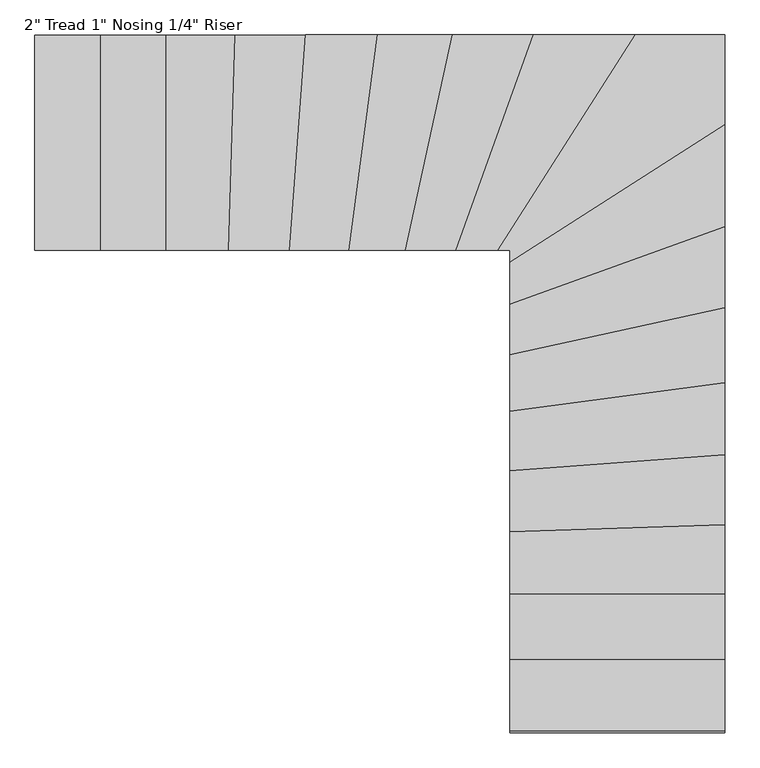
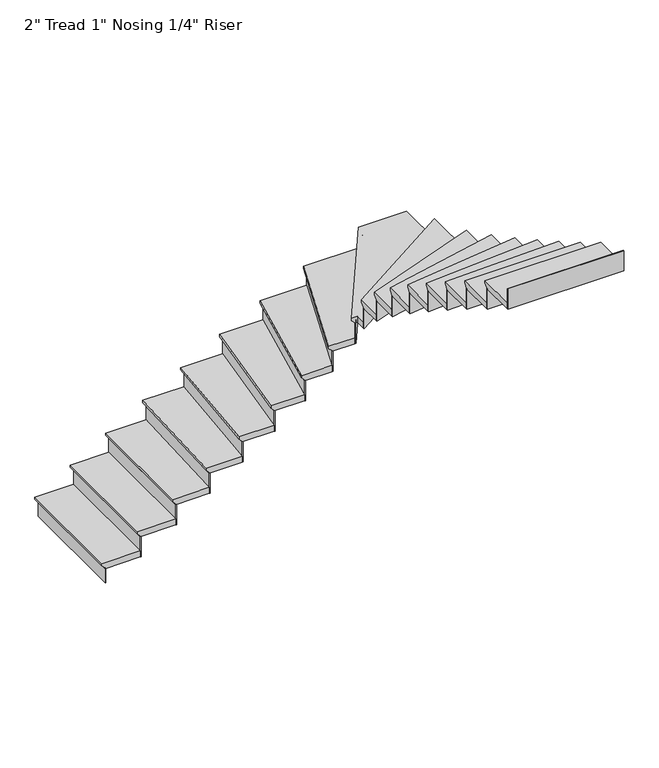
"""IFC4 building model written with IfcOpenShell, lengths in millimetres: stair flight geometry."""

from ifc_helpers import new_model, si_unit, origin, place, context, project, spatial, faceted_brep, source, transform, mapped, element, save


def stair_flight_aca28aa2(model_context):
    return source(origin(), model_context, "Body", "Brep", [
        faceted_brep([(-5670.2346501, 6411.0271763, 150.2833333), (-5670.2346501, 6411.0271763, 169.3333333), (-5670.2346501, 7325.4271763, 169.3333333), (-5670.2346501, 7325.4271763, 150.2833333), (-5644.8346501, 6411.0271763, 124.8833333), (-5644.8346501, 7325.4271763, 124.8833333), (-5365.4346501, 6411.0271763, 169.3333333), (-5365.4346501, 7325.4271763, 169.3333333), (-5644.8346501, 7325.4271763, 118.5333333), (-5365.4346501, 7325.4271763, 118.5333333), (-5365.4346501, 6411.0271763, 118.5333333), (-5644.8346501, 6411.0271763, 118.5333333)], [[[0, 1, 2, 3]], [[4, 0, 3, 5]], [[2, 1, 6, 7]], [[8, 9, 10, 11]], [[2, 7, 9, 8, 5, 3]], [[8, 11, 4, 5]], [[6, 1, 0, 4, 11, 10]], [[7, 6, 10, 9]]]),
        faceted_brep([(-5644.8346501, 6411.0271763, 118.5333333), (-5644.8346501, 6411.0271763, 0.0), (-5638.4846501, 6411.0271763, 0.0), (-5638.4846501, 6411.0271763, 118.5333333), (-5644.8346501, 7325.4271763, 118.5333333), (-5638.4846501, 7325.4271763, 118.5333333), (-5638.4846501, 7325.4271763, 0.0), (-5644.8346501, 7325.4271763, 0.0)], [[[0, 1, 2, 3]], [[4, 5, 6, 7]], [[1, 0, 4, 7]], [[2, 1, 7, 6]], [[3, 2, 6, 5]], [[0, 3, 5, 4]]]),
        faceted_brep([(-5365.4346501, 6411.0271763, 287.8666667), (-5365.4346501, 6411.0271763, 118.5333333), (-5359.0846501, 6411.0271763, 118.5333333), (-5359.0846501, 6411.0271763, 287.8666667), (-5365.4346501, 7325.4271763, 287.8666667), (-5359.0846501, 7325.4271763, 287.8666667), (-5359.0846501, 7325.4271763, 118.5333333), (-5365.4346501, 7325.4271763, 118.5333333)], [[[0, 1, 2, 3]], [[4, 5, 6, 7]], [[1, 0, 4, 7]], [[2, 1, 7, 6]], [[3, 2, 6, 5]], [[0, 3, 5, 4]]]),
        faceted_brep([(-5390.8346501, 7325.4271763, 338.6666667), (-5390.8346501, 6411.0271763, 338.6666667), (-5086.0346501, 6411.0271763, 338.6666667), (-5086.0346501, 7325.4271763, 338.6666667), (-5365.4346501, 7325.4271763, 287.8666667), (-5086.0346501, 7325.4271763, 287.8666667), (-5086.0346501, 6411.0271763, 287.8666667), (-5365.4346501, 6411.0271763, 287.8666667), (-5365.4346501, 7325.4271763, 294.2166667), (-5390.8346501, 7325.4271763, 319.6166667), (-5365.4346501, 6411.0271763, 294.2166667), (-5390.8346501, 6411.0271763, 319.6166667)], [[[0, 1, 2, 3]], [[4, 5, 6, 7]], [[0, 3, 5, 4, 8, 9]], [[4, 7, 10, 8]], [[2, 1, 11, 10, 7, 6]], [[3, 2, 6, 5]], [[11, 1, 0, 9]], [[10, 11, 9, 8]]]),
        faceted_brep([(-5086.0346501, 6411.0271763, 457.2), (-5086.0346501, 6411.0271763, 287.8666667), (-5079.6846501, 6411.0271763, 287.8666667), (-5079.6846501, 6411.0271763, 457.2), (-5086.0346501, 7325.4271763, 457.2), (-5079.6846501, 7325.4271763, 457.2), (-5079.6846501, 7325.4271763, 287.8666667), (-5086.0346501, 7325.4271763, 287.8666667)], [[[0, 1, 2, 3]], [[4, 5, 6, 7]], [[1, 0, 4, 7]], [[2, 1, 7, 6]], [[3, 2, 6, 5]], [[0, 3, 5, 4]]]),
        faceted_brep([(-5111.4346501, 7325.4271763, 508.0), (-5111.4346501, 6411.0271763, 508.0), (-4821.1765248, 6411.0271763, 508.0), (-4792.0670407, 7325.4271763, 508.0), (-5086.0346501, 7325.4271763, 457.2), (-4792.0670407, 7325.4271763, 457.2), (-4821.1765248, 6411.0271763, 457.2), (-5086.0346501, 6411.0271763, 457.2), (-5086.0346501, 7325.4271763, 463.55), (-5111.4346501, 7325.4271763, 488.95), (-5086.0346501, 6411.0271763, 463.55), (-5111.4346501, 6411.0271763, 488.95)], [[[0, 1, 2, 3]], [[4, 5, 6, 7]], [[0, 3, 5, 4, 8, 9]], [[4, 7, 10, 8]], [[2, 1, 11, 10, 7, 6]], [[3, 2, 6, 5]], [[11, 1, 0, 9]], [[10, 11, 9, 8]]]),
        faceted_brep([(-4821.1765248, 6411.0271763, 626.5333333), (-4821.1765248, 6411.0271763, 457.2), (-4814.823308, 6411.0271763, 457.2), (-4814.823308, 6411.0271763, 626.5333333), (-4792.0670407, 7325.4271763, 626.5333333), (-4785.7138239, 7325.4271763, 626.5333333), (-4785.7138239, 7325.4271763, 457.2), (-4792.0670407, 7325.4271763, 457.2)], [[[0, 1, 2, 3]], [[4, 5, 6, 7]], [[1, 0, 4, 7]], [[2, 1, 7, 6]], [[3, 2, 6, 5]], [[0, 3, 5, 4]]]),
        faceted_brep([(-4817.4799081, 7325.4271763, 677.3333333), (-4846.5893922, 6411.0271763, 677.3333333), (-4560.9843582, 6411.0271763, 677.3333333), (-4493.3461539, 7325.4271763, 677.3333333), (-4792.0670407, 7325.4271763, 626.5333333), (-4493.3461539, 7325.4271763, 626.5333333), (-4560.9843582, 6411.0271763, 626.5333333), (-4821.1765248, 6411.0271763, 626.5333333), (-4792.0670407, 7325.4271763, 632.8833333), (-4817.4799081, 7325.4271763, 658.2833333), (-4821.1765248, 6411.0271763, 632.8833333), (-4846.5893922, 6411.0271763, 658.2833333)], [[[0, 1, 2, 3]], [[4, 5, 6, 7]], [[0, 3, 5, 4, 8, 9]], [[4, 7, 10, 8]], [[2, 1, 11, 10, 7, 6]], [[3, 2, 6, 5]], [[11, 1, 0, 9]], [[10, 11, 9, 8]]]),
        faceted_brep([(-4560.9843582, 6411.0271763, 795.8666667), (-4560.9843582, 6411.0271763, 626.5333333), (-4554.6170096, 6411.0271763, 626.5333333), (-4554.6170096, 6411.0271763, 795.8666667), (-4493.3461539, 7325.4271763, 795.8666667), (-4486.9788054, 7325.4271763, 795.8666667), (-4486.9788054, 7325.4271763, 626.5333333), (-4493.3461539, 7325.4271763, 626.5333333)], [[[0, 1, 2, 3]], [[4, 5, 6, 7]], [[1, 0, 4, 7]], [[2, 1, 7, 6]], [[3, 2, 6, 5]], [[0, 3, 5, 4]]]),
        faceted_brep([(-4518.815548, 7325.4271763, 846.6666667), (-4586.4537523, 6411.0271763, 846.6666667), (-4308.1332907, 6411.0271763, 846.6666667), (-4187.0928787, 7325.4271763, 846.6666667), (-4493.3461539, 7325.4271763, 795.8666667), (-4187.0928787, 7325.4271763, 795.8666667), (-4308.1332907, 6411.0271763, 795.8666667), (-4560.9843582, 6411.0271763, 795.8666667), (-4493.3461539, 7325.4271763, 802.2166667), (-4518.815548, 7325.4271763, 827.6166667), (-4560.9843582, 6411.0271763, 802.2166667), (-4586.4537523, 6411.0271763, 827.6166667)], [[[0, 1, 2, 3]], [[4, 5, 6, 7]], [[0, 3, 5, 4, 8, 9]], [[4, 7, 10, 8]], [[2, 1, 11, 10, 7, 6]], [[3, 2, 6, 5]], [[11, 1, 0, 9]], [[10, 11, 9, 8]]]),
        faceted_brep([(-4308.1332907, 6411.0271763, 965.2), (-4308.1332907, 6411.0271763, 795.8666667), (-4301.7278994, 6411.0271763, 795.8666667), (-4301.7278994, 6411.0271763, 965.2), (-4187.0928787, 7325.4271763, 965.2), (-4180.6874873, 7325.4271763, 965.2), (-4180.6874873, 7325.4271763, 795.8666667), (-4187.0928787, 7325.4271763, 795.8666667)], [[[0, 1, 2, 3]], [[4, 5, 6, 7]], [[1, 0, 4, 7]], [[2, 1, 7, 6]], [[3, 2, 6, 5]], [[0, 3, 5, 4]]]),
        faceted_brep([(-4212.7144441, 7325.4271763, 1016.0), (-4333.7548562, 6411.0271763, 1016.0), (-4067.8285854, 6411.0271763, 1016.0), (-3867.8399188, 7325.4271763, 1016.0), (-4187.0928787, 7325.4271763, 965.2), (-3867.8399188, 7325.4271763, 965.2), (-4067.8285854, 6411.0271763, 965.2), (-4308.1332907, 6411.0271763, 965.2), (-4187.0928787, 7325.4271763, 971.55), (-4212.7144441, 7325.4271763, 996.95), (-4308.1332907, 6411.0271763, 971.55), (-4333.7548562, 6411.0271763, 996.95)], [[[0, 1, 2, 3]], [[4, 5, 6, 7]], [[0, 3, 5, 4, 8, 9]], [[4, 7, 10, 8]], [[2, 1, 11, 10, 7, 6]], [[3, 2, 6, 5]], [[11, 1, 0, 9]], [[10, 11, 9, 8]]]),
        faceted_brep([(-4067.8285854, 6411.0271763, 1134.5333333), (-4067.8285854, 6411.0271763, 965.2), (-4061.3284859, 6411.0271763, 965.2), (-4061.3284859, 6411.0271763, 1134.5333333), (-3867.8399188, 7325.4271763, 1134.5333333), (-3861.3398193, 7325.4271763, 1134.5333333), (-3861.3398193, 7325.4271763, 965.2), (-3867.8399188, 7325.4271763, 965.2)], [[[0, 1, 2, 3]], [[4, 5, 6, 7]], [[1, 0, 4, 7]], [[2, 1, 7, 6]], [[3, 2, 6, 5]], [[0, 3, 5, 4]]]),
        faceted_brep([(-3893.8403168, 7325.4271763, 1185.3333333), (-4093.8289834, 6411.0271763, 1185.3333333), (-3851.7328226, 6411.0271763, 1185.3333333), (-3523.1563179, 7325.4271763, 1185.3333333), (-3867.8399188, 7325.4271763, 1134.5333333), (-3523.1563179, 7325.4271763, 1134.5333333), (-3851.7328226, 6411.0271763, 1134.5333333), (-4067.8285854, 6411.0271763, 1134.5333333), (-3867.8399188, 7325.4271763, 1140.8833333), (-3893.8403168, 7325.4271763, 1166.2833333), (-4067.8285854, 6411.0271763, 1140.8833333), (-4093.8289834, 6411.0271763, 1166.2833333)], [[[0, 1, 2, 3]], [[4, 5, 6, 7]], [[0, 3, 5, 4, 8, 9]], [[4, 7, 10, 8]], [[2, 1, 11, 10, 7, 6]], [[3, 2, 6, 5]], [[11, 1, 0, 9]], [[10, 11, 9, 8]]]),
        faceted_brep([(-3851.7328226, 6411.0271763, 1303.8666667), (-3851.7328226, 6411.0271763, 1134.5333333), (-3844.9853027, 6411.0271763, 1134.5333333), (-3844.9853027, 6411.0271763, 1303.8666667), (-3523.1563179, 7325.4271763, 1303.8666667), (-3516.4087979, 7325.4271763, 1303.8666667), (-3516.4087979, 7325.4271763, 1134.5333333), (-3523.1563179, 7325.4271763, 1134.5333333)], [[[0, 1, 2, 3]], [[4, 5, 6, 7]], [[1, 0, 4, 7]], [[2, 1, 7, 6]], [[3, 2, 6, 5]], [[0, 3, 5, 4]]]),
        faceted_brep([(-3550.1463978, 7325.4271763, 1354.6666667), (-3878.7229025, 6411.0271763, 1354.6666667), (-3669.4620272, 6411.0271763, 1354.6666667), (-3084.8625918, 7325.4271763, 1354.6666667), (-3523.1563179, 7325.4271763, 1303.8666667), (-3084.8625918, 7325.4271763, 1303.8666667), (-3669.4620272, 6411.0271763, 1303.8666667), (-3851.7328226, 6411.0271763, 1303.8666667), (-3523.1563179, 7325.4271763, 1310.2166667), (-3550.1463978, 7325.4271763, 1335.6166667), (-3851.7328226, 6411.0271763, 1310.2166667), (-3878.7229025, 6411.0271763, 1335.6166667)], [[[0, 1, 2, 3]], [[4, 5, 6, 7]], [[0, 3, 5, 4, 8, 9]], [[4, 7, 10, 8]], [[2, 1, 11, 10, 7, 6]], [[3, 2, 6, 5]], [[11, 1, 0, 9]], [[10, 11, 9, 8]]]),
        faceted_brep([(-3669.4620272, 6411.0271763, 1473.2), (-3669.4620272, 6411.0271763, 1303.8666667), (-3661.9251968, 6411.0271763, 1303.8666667), (-3661.9251968, 6411.0271763, 1473.2), (-3084.8625918, 7325.4271763, 1473.2), (-3077.3257614, 7325.4271763, 1473.2), (-3077.3257614, 7325.4271763, 1303.8666667), (-3084.8625918, 7325.4271763, 1303.8666667)], [[[0, 1, 2, 3]], [[4, 5, 6, 7]], [[1, 0, 4, 7]], [[2, 1, 7, 6]], [[3, 2, 6, 5]], [[0, 3, 5, 4]]]),
        faceted_brep([(-2734.2976606, 6914.5676018, 1524.0), (-2734.2976606, 7325.4271763, 1524.0), (-3115.0099135, 7325.4271763, 1524.0), (-3699.6093489, 6411.0271763, 1524.0), (-3648.6976606, 6411.0271763, 1524.0), (-3648.6976606, 6329.9681664, 1524.0), (-2734.2976606, 7325.4271763, 1473.2), (-2734.2976606, 6914.5676018, 1473.2), (-3648.6976606, 6329.9681664, 1473.2), (-3648.6976606, 6411.0271763, 1473.2), (-3669.4620272, 6411.0271763, 1473.2), (-3084.8625918, 7325.4271763, 1473.2), (-3084.8625918, 7325.4271763, 1479.55), (-3115.0099135, 7325.4271763, 1504.95), (-3669.4620272, 6411.0271763, 1479.55), (-3699.6093489, 6411.0271763, 1504.95)], [[[0, 1, 2, 3, 4, 5]], [[6, 7, 8, 9, 10, 11]], [[1, 0, 7, 6]], [[2, 1, 6, 11, 12, 13]], [[11, 10, 14, 12]], [[4, 3, 15, 14, 10, 9]], [[5, 4, 9, 8]], [[0, 5, 8, 7]], [[15, 3, 2, 13]], [[14, 15, 13, 12]]]),
        faceted_brep([(-3648.6976606, 6329.9681664, 1642.5333333), (-3648.6976606, 6329.9681664, 1473.2), (-3648.6976606, 6322.4313359, 1473.2), (-3648.6976606, 6322.4313359, 1642.5333333), (-2734.2976606, 6914.5676018, 1642.5333333), (-2734.2976606, 6907.0307714, 1642.5333333), (-2734.2976606, 6907.0307714, 1473.2), (-2734.2976606, 6914.5676018, 1473.2)], [[[0, 1, 2, 3]], [[4, 5, 6, 7]], [[1, 0, 4, 7]], [[2, 1, 7, 6]], [[3, 2, 6, 5]], [[0, 3, 5, 4]]]),
        faceted_brep([(-2734.2976606, 6944.7149234, 1693.3333333), (-3648.6976606, 6360.115488, 1693.3333333), (-3648.6976606, 6154.0118545, 1693.3333333), (-2734.2976606, 6482.5883593, 1693.3333333), (-2734.2976606, 6914.5676018, 1642.5333333), (-2734.2976606, 6482.5883593, 1642.5333333), (-3648.6976606, 6154.0118545, 1642.5333333), (-3648.6976606, 6329.9681664, 1642.5333333), (-2734.2976606, 6914.5676018, 1648.8833333), (-2734.2976606, 6944.7149234, 1674.2833333), (-3648.6976606, 6329.9681664, 1648.8833333), (-3648.6976606, 6360.115488, 1674.2833333)], [[[0, 1, 2, 3]], [[4, 5, 6, 7]], [[0, 3, 5, 4, 8, 9]], [[4, 7, 10, 8]], [[2, 1, 11, 10, 7, 6]], [[3, 2, 6, 5]], [[11, 1, 0, 9]], [[10, 11, 9, 8]]]),
        faceted_brep([(-3648.6976606, 6154.0118545, 1811.8666667), (-3648.6976606, 6154.0118545, 1642.5333333), (-3648.6976606, 6147.2643345, 1642.5333333), (-3648.6976606, 6147.2643345, 1811.8666667), (-2734.2976606, 6482.5883593, 1811.8666667), (-2734.2976606, 6475.8408393, 1811.8666667), (-2734.2976606, 6475.8408393, 1642.5333333), (-2734.2976606, 6482.5883593, 1642.5333333)], [[[0, 1, 2, 3]], [[4, 5, 6, 7]], [[1, 0, 4, 7]], [[2, 1, 7, 6]], [[3, 2, 6, 5]], [[0, 3, 5, 4]]]),
        faceted_brep([(-2734.2976606, 6509.5784392, 1862.6666667), (-3648.6976606, 6181.0019344, 1862.6666667), (-3648.6976606, 5939.8954554, 1862.6666667), (-2734.2976606, 6139.884122, 1862.6666667), (-2734.2976606, 6482.5883593, 1811.8666667), (-2734.2976606, 6139.884122, 1811.8666667), (-3648.6976606, 5939.8954554, 1811.8666667), (-3648.6976606, 6154.0118545, 1811.8666667), (-2734.2976606, 6482.5883593, 1818.2166667), (-2734.2976606, 6509.5784392, 1843.6166667), (-3648.6976606, 6154.0118545, 1818.2166667), (-3648.6976606, 6181.0019344, 1843.6166667)], [[[0, 1, 2, 3]], [[4, 5, 6, 7]], [[0, 3, 5, 4, 8, 9]], [[4, 7, 10, 8]], [[2, 1, 11, 10, 7, 6]], [[3, 2, 6, 5]], [[11, 1, 0, 9]], [[10, 11, 9, 8]]]),
        faceted_brep([(-3648.6976606, 5939.8954554, 1981.2), (-3648.6976606, 5939.8954554, 1811.8666667), (-3648.6976606, 5933.3953559, 1811.8666667), (-3648.6976606, 5933.3953559, 1981.2), (-2734.2976606, 6139.884122, 1981.2), (-2734.2976606, 6133.3840225, 1981.2), (-2734.2976606, 6133.3840225, 1811.8666667), (-2734.2976606, 6139.884122, 1811.8666667)], [[[0, 1, 2, 3]], [[4, 5, 6, 7]], [[1, 0, 4, 7]], [[2, 1, 7, 6]], [[3, 2, 6, 5]], [[0, 3, 5, 4]]]),
        faceted_brep([(-2734.2976606, 6165.8845201, 2032.0), (-3648.6976606, 5965.8958535, 2032.0), (-3648.6976606, 5700.3484153, 2032.0), (-2734.2976606, 5821.3888274, 2032.0), (-2734.2976606, 6139.884122, 1981.2), (-2734.2976606, 5821.3888274, 1981.2), (-3648.6976606, 5700.3484153, 1981.2), (-3648.6976606, 5939.8954554, 1981.2), (-2734.2976606, 6139.884122, 1987.55), (-2734.2976606, 6165.8845201, 2012.95), (-3648.6976606, 5939.8954554, 1987.55), (-3648.6976606, 5965.8958535, 2012.95)], [[[0, 1, 2, 3]], [[4, 5, 6, 7]], [[0, 3, 5, 4, 8, 9]], [[4, 7, 10, 8]], [[2, 1, 11, 10, 7, 6]], [[3, 2, 6, 5]], [[11, 1, 0, 9]], [[10, 11, 9, 8]]]),
        faceted_brep([(-3648.6976606, 5700.3484153, 2150.5333333), (-3648.6976606, 5700.3484153, 1981.2), (-3648.6976606, 5693.9430239, 1981.2), (-3648.6976606, 5693.9430239, 2150.5333333), (-2734.2976606, 5821.3888274, 2150.5333333), (-2734.2976606, 5814.983436, 2150.5333333), (-2734.2976606, 5814.983436, 1981.2), (-2734.2976606, 5821.3888274, 1981.2)], [[[0, 1, 2, 3]], [[4, 5, 6, 7]], [[1, 0, 4, 7]], [[2, 1, 7, 6]], [[3, 2, 6, 5]], [[0, 3, 5, 4]]]),
        faceted_brep([(-2734.2976606, 5847.0103928, 2201.3333333), (-3648.6976606, 5725.9699807, 2201.3333333), (-3648.6976606, 5447.8016905, 2201.3333333), (-2734.2976606, 5515.4398948, 2201.3333333), (-2734.2976606, 5821.3888274, 2150.5333333), (-2734.2976606, 5515.4398948, 2150.5333333), (-3648.6976606, 5447.8016905, 2150.5333333), (-3648.6976606, 5700.3484153, 2150.5333333), (-2734.2976606, 5821.3888274, 2156.8833333), (-2734.2976606, 5847.0103928, 2182.2833333), (-3648.6976606, 5700.3484153, 2156.8833333), (-3648.6976606, 5725.9699807, 2182.2833333)], [[[0, 1, 2, 3]], [[4, 5, 6, 7]], [[0, 3, 5, 4, 8, 9]], [[4, 7, 10, 8]], [[2, 1, 11, 10, 7, 6]], [[3, 2, 6, 5]], [[11, 1, 0, 9]], [[10, 11, 9, 8]]]),
        faceted_brep([(-3648.6976606, 5447.8016905, 2319.8666667), (-3648.6976606, 5447.8016905, 2150.5333333), (-3648.6976606, 5441.434342, 2150.5333333), (-3648.6976606, 5441.434342, 2319.8666667), (-2734.2976606, 5515.4398948, 2319.8666667), (-2734.2976606, 5509.0725463, 2319.8666667), (-2734.2976606, 5509.0725463, 2150.5333333), (-2734.2976606, 5515.4398948, 2150.5333333)], [[[0, 1, 2, 3]], [[4, 5, 6, 7]], [[1, 0, 4, 7]], [[2, 1, 7, 6]], [[3, 2, 6, 5]], [[0, 3, 5, 4]]]),
        faceted_brep([(-2734.2976606, 5540.9092889, 2370.6666667), (-3648.6976606, 5473.2710846, 2370.6666667), (-3648.6976606, 5187.7225773, 2370.6666667), (-2734.2976606, 5216.8320614, 2370.6666667), (-2734.2976606, 5515.4398948, 2319.8666667), (-2734.2976606, 5216.8320614, 2319.8666667), (-3648.6976606, 5187.7225773, 2319.8666667), (-3648.6976606, 5447.8016905, 2319.8666667), (-2734.2976606, 5515.4398948, 2326.2166667), (-2734.2976606, 5540.9092889, 2351.6166667), (-3648.6976606, 5447.8016905, 2326.2166667), (-3648.6976606, 5473.2710846, 2351.6166667)], [[[0, 1, 2, 3]], [[4, 5, 6, 7]], [[0, 3, 5, 4, 8, 9]], [[4, 7, 10, 8]], [[2, 1, 11, 10, 7, 6]], [[3, 2, 6, 5]], [[11, 1, 0, 9]], [[10, 11, 9, 8]]]),
        faceted_brep([(-3648.6976606, 5187.7225773, 2489.2), (-3648.6976606, 5187.7225773, 2319.8666667), (-3648.6976606, 5181.3693605, 2319.8666667), (-3648.6976606, 5181.3693605, 2489.2), (-2734.2976606, 5216.8320614, 2489.2), (-2734.2976606, 5210.4788446, 2489.2), (-2734.2976606, 5210.4788446, 2319.8666667), (-2734.2976606, 5216.8320614, 2319.8666667)], [[[0, 1, 2, 3]], [[4, 5, 6, 7]], [[1, 0, 4, 7]], [[2, 1, 7, 6]], [[3, 2, 6, 5]], [[0, 3, 5, 4]]]),
        faceted_brep([(-2734.2976606, 5242.2449288, 2540.0), (-3648.6976606, 5213.1354447, 2540.0), (-3648.6976606, 4922.8901868, 2540.0), (-2734.2976606, 4922.8901868, 2540.0), (-2734.2976606, 5216.8320614, 2489.2), (-2734.2976606, 4922.8901868, 2489.2), (-3648.6976606, 4922.8901868, 2489.2), (-3648.6976606, 5187.7225773, 2489.2), (-2734.2976606, 5216.8320614, 2495.55), (-2734.2976606, 5242.2449288, 2520.95), (-3648.6976606, 5187.7225773, 2495.55), (-3648.6976606, 5213.1354447, 2520.95)], [[[0, 1, 2, 3]], [[4, 5, 6, 7]], [[0, 3, 5, 4, 8, 9]], [[4, 7, 10, 8]], [[2, 1, 11, 10, 7, 6]], [[3, 2, 6, 5]], [[11, 1, 0, 9]], [[10, 11, 9, 8]]]),
        faceted_brep([(-3648.6976606, 4922.8901868, 2658.5333333), (-3648.6976606, 4922.8901868, 2489.2), (-3648.6976606, 4916.5401868, 2489.2), (-3648.6976606, 4916.5401868, 2658.5333333), (-2734.2976606, 4922.8901868, 2658.5333333), (-2734.2976606, 4916.5401868, 2658.5333333), (-2734.2976606, 4916.5401868, 2489.2), (-2734.2976606, 4922.8901868, 2489.2)], [[[0, 1, 2, 3]], [[4, 5, 6, 7]], [[1, 0, 4, 7]], [[2, 1, 7, 6]], [[3, 2, 6, 5]], [[0, 3, 5, 4]]]),
        faceted_brep([(-2734.2976606, 4948.2901868, 2709.3333333), (-3648.6976606, 4948.2901868, 2709.3333333), (-3648.6976606, 4643.4901868, 2709.3333333), (-2734.2976606, 4643.4901868, 2709.3333333), (-2734.2976606, 4922.8901868, 2658.5333333), (-2734.2976606, 4643.4901868, 2658.5333333), (-3648.6976606, 4643.4901868, 2658.5333333), (-3648.6976606, 4922.8901868, 2658.5333333), (-2734.2976606, 4922.8901868, 2664.8833333), (-2734.2976606, 4948.2901868, 2690.2833333), (-3648.6976606, 4922.8901868, 2664.8833333), (-3648.6976606, 4948.2901868, 2690.2833333)], [[[0, 1, 2, 3]], [[4, 5, 6, 7]], [[0, 3, 5, 4, 8, 9]], [[4, 7, 10, 8]], [[2, 1, 11, 10, 7, 6]], [[3, 2, 6, 5]], [[11, 1, 0, 9]], [[10, 11, 9, 8]]]),
        faceted_brep([(-3648.6976606, 4643.4901868, 2827.8666667), (-3648.6976606, 4643.4901868, 2658.5333333), (-3648.6976606, 4637.1401868, 2658.5333333), (-3648.6976606, 4637.1401868, 2827.8666667), (-2734.2976606, 4643.4901868, 2827.8666667), (-2734.2976606, 4637.1401868, 2827.8666667), (-2734.2976606, 4637.1401868, 2658.5333333), (-2734.2976606, 4643.4901868, 2658.5333333)], [[[0, 1, 2, 3]], [[4, 5, 6, 7]], [[1, 0, 4, 7]], [[2, 1, 7, 6]], [[3, 2, 6, 5]], [[0, 3, 5, 4]]]),
        faceted_brep([(-3648.6976606, 4364.0901868, 2997.2), (-3648.6976606, 4364.0901868, 2827.8666667), (-3648.6976606, 4357.7401868, 2827.8666667), (-3648.6976606, 4357.7401868, 2997.2), (-2734.2976606, 4364.0901868, 2997.2), (-2734.2976606, 4357.7401868, 2997.2), (-2734.2976606, 4357.7401868, 2827.8666667), (-2734.2976606, 4364.0901868, 2827.8666667)], [[[0, 1, 2, 3]], [[4, 5, 6, 7]], [[1, 0, 4, 7]], [[2, 1, 7, 6]], [[3, 2, 6, 5]], [[0, 3, 5, 4]]]),
        faceted_brep([(-2734.2976606, 4668.8901868, 2878.6666667), (-3648.6976606, 4668.8901868, 2878.6666667), (-3648.6976606, 4364.0901868, 2878.6666667), (-2734.2976606, 4364.0901868, 2878.6666667), (-2734.2976606, 4643.4901868, 2827.8666667), (-2734.2976606, 4364.0901868, 2827.8666667), (-3648.6976606, 4364.0901868, 2827.8666667), (-3648.6976606, 4643.4901868, 2827.8666667), (-2734.2976606, 4643.4901868, 2834.2166667), (-2734.2976606, 4668.8901868, 2859.6166667), (-3648.6976606, 4643.4901868, 2834.2166667), (-3648.6976606, 4668.8901868, 2859.6166667)], [[[0, 1, 2, 3]], [[4, 5, 6, 7]], [[0, 3, 5, 4, 8, 9]], [[4, 7, 10, 8]], [[2, 1, 11, 10, 7, 6]], [[3, 2, 6, 5]], [[11, 1, 0, 9]], [[10, 11, 9, 8]]]),
    ])


if __name__ == "__main__":
    model = new_model("IFC4")
    model_context = context("Model", 3, world=origin())
    ifc_project = project(units=[si_unit("LENGTHUNIT", "METRE", prefix="MILLI")], contexts=[model_context])
    site = spatial("IfcSite", under=ifc_project)
    building = spatial("IfcBuilding", under=site)
    placement = place(None, origin())
    stair_flight_shape = stair_flight_aca28aa2(model_context)
    element("IfcStairFlight", 1, ObjectType="2\" Tread 1\" Nosing 1/4\" Riser", at=placement, inside=building, context=model_context, shape_type="MappedRepresentation", body=[
        mapped(stair_flight_shape, transform((0.0, 0.0, 0.0), x_axis=(1.0, 0.0, 0.0), y_axis=(0.0, 1.0, 0.0), z_axis=(0.0, 0.0, 1.0))),
    ])
    save(model, "model.ifc")
